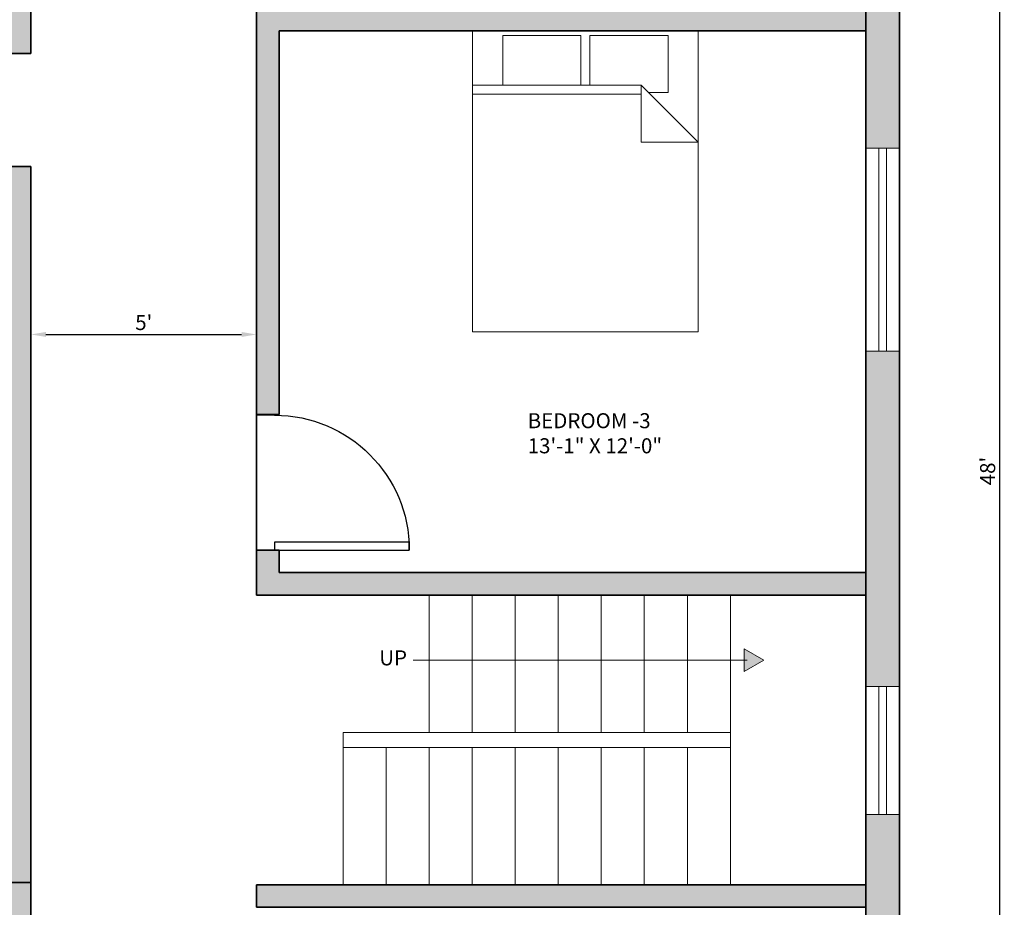
# Model space of a CAD drawing. Units: inches. Extents: x -91 to 518, y -600 to 105.
# Tile 3 of 4: x 248 to 509, y -391 to -155. Entities that reach past the tile are written whole.
import ezdxf

# ---------------------------------------------------------------- set-up
doc = ezdxf.new("R2010")
doc.units = ezdxf.units.IN
for name, color, linetype, lineweight in [('A-ANNO-DIMS', 2, 'Continuous', 18), ('A-ANNO-SYMB', 7, 'Continuous', 18), ('A-ANNO-TEXT', 7, 'Continuous', 18), ('A-AREA-IDEN', 7, 'Continuous', 18), ('A-DOOR', 4, 'Continuous', 25), ('A-FLOR-STRS', 7, 'Continuous', 18), ('A-FURN', 8, 'Continuous', 18), ('A-GLAZ', 6, 'Continuous', 18), ('A-WALL', 7, 'Continuous', 35), ('A-WALL-PATT', 251, 'Continuous', 13)]:
    doc.layers.add(name, color=color, linetype=linetype, lineweight=lineweight)
doc.styles.get("Standard").update_dxf_attribs({"font": 'arial.ttf'})
doc.dimstyles.new('ISO-25', dxfattribs={"dimtxt": 4, "dimasz": 4, "dimexe": 1.25, "dimexo": 0.625, "dimtad": 1, "dimlunit": 3, "dimtxsty": 'Standard', "dimcen": 2.5, "dimadec": 0, "dimazin": 0, "dimtfac": 1, "dimtmove": 0, "dimatfit": 3, "dimfxl": 1, "dimfxlon": 1, "dimarcsym": 0})

# ---------------------------------------------------------------- blocks, each defined once
blk = doc.blocks.new('*U2')
for p, q in [((0, 0), (0, -100)), ((750, 0), (750, -100))]:
    blk.add_line(p, q)
blk.add_lwpolyline([(0, 0), (0, 750), (43.75, 750), (43.75, 0)], close=True)
blk.add_arc((0, 0), 750, 0, 90)
blk = doc.blocks.new('Bed - Queen')
for p, q in [((0, -80.00003), (0, 0)), ((0, 0), (59.99999, 0)), ((59.99999, 0), (59.99999, -80.00003)), ((7.99999, -1.2), (28.79998, -1.2)), ((7.99999, -14.4), (7.99999, -1.2)), ((28.79998, -1.2), (28.79998, -14.4)), ((31.19999, -1.2), (51.99999, -1.2)), ((31.19999, -14.4), (31.19999, -1.2)), ((51.99999, -1.2), (51.99999, -16.4)), ((0, -14.4), (44.8, -14.4)), ((59.99999, -29.6), (44.8, -14.4)), ((44.8, -14.4), (44.8, -29.6)), ((44.8, -16.8), (0, -16.8)), ((51.99999, -16.4), (46.79936, -16.4)), ((44.8, -29.6), (59.99999, -29.6)), ((59.99999, -80.00003), (0, -80.00003))]:
    blk.add_line(p, q)
blk = doc.blocks.new('*D8')
at = {"layer": 'A-ANNO-DIMS', "color": 0, "lineweight": -2, "transparency": 16777216}
for p, q in [((250.54, -239), (250.54, -237.75)), ((310.54, -239), (310.54, -237.75)), ((254.54, -239), (306.54, -239))]:
    blk.add_line(p, q, dxfattribs=at)
at = {"layer": 'A-ANNO-DIMS', "color": 0, "transparency": 16777216}
for points in [[(254.54, -238.33), (254.54, -239.66), (250.54, -239)], [(306.54, -238.33), (306.54, -239.66), (310.54, -239)]]:
    blk.add_solid(points, dxfattribs=at)
at = {"layer": 'Defpoints', "color": 0, "transparency": 16777216}
for p in [(250.54, -239), (310.54, -239), (310.54, -239)]:
    blk.add_point(p, dxfattribs=at)
at = {"layer": 'A-ANNO-DIMS', "color": 0, "transparency": 16777216, "insert": (280.54, -236.34), "char_height": 4, "attachment_point": 5}
blk.add_mtext("5'", dxfattribs=at)
blk = doc.blocks.new('*D10')
at = {"layer": 'A-ANNO-DIMS', "color": 0, "lineweight": -2, "transparency": 16777216}
for p, q in [((507.14, 12.69), (509.39, 12.69)), ((508.14, 8.69), (508.14, -559.31)), ((507.14, -563.31), (509.39, -563.31))]:
    blk.add_line(p, q, dxfattribs=at)
at = {"layer": 'A-ANNO-DIMS', "color": 0, "transparency": 16777216}
for points in [[(507.48, 8.69), (508.81, 8.69), (508.14, 12.69)], [(507.48, -559.31), (508.81, -559.31), (508.14, -563.31)]]:
    blk.add_solid(points, dxfattribs=at)
at = {"layer": 'Defpoints', "color": 0, "transparency": 16777216}
for p in [(481.54, 12.69), (481.54, -563.31), (508.14, -563.31)]:
    blk.add_point(p, dxfattribs=at)
at = {"layer": 'A-ANNO-DIMS', "color": 0, "transparency": 16777216, "insert": (505.48, -275.31), "char_height": 4, "attachment_point": 5, "rotation": 90}
blk.add_mtext("48'", dxfattribs=at)
blk = doc.blocks.new('WIN-54IN')
for p, q in [((0, 5.5), (54, 5.5)), ((0, 3.5), (54, 3.5))]:
    blk.add_line(p, q)
blk.add_lwpolyline([(0, 9), (54, 9), (54, 0), (0, 0)], close=True)
blk = doc.blocks.new('WIN-34IN')
for p, q in [((0, 5.5), (34, 5.5)), ((0, 3.5), (34, 3.5))]:
    blk.add_line(p, q)
blk.add_lwpolyline([(0, 9), (34, 9), (34, 0), (0, 0)], close=True)
blk = doc.blocks.new('*D35')
at = {"layer": 'A-ANNO-DIMS', "color": 0, "lineweight": -2, "transparency": 16777216}
for p, q in [((-81.99, -381.31), (-81.99, -377.31)), ((-80.99, -385.31), (-83.24, -385.31)), ((-81.99, -385.31), (-81.99, -391.31)), ((-80.99, -391.31), (-83.24, -391.31)), ((-81.99, -395.31), (-81.99, -411.19))]:
    blk.add_line(p, q, dxfattribs=at)
at = {"layer": 'A-ANNO-DIMS', "color": 0, "transparency": 16777216}
for points in [[(-82.66, -381.31), (-81.32, -381.31), (-81.99, -385.31)], [(-82.66, -395.31), (-81.32, -395.31), (-81.99, -391.31)]]:
    blk.add_solid(points, dxfattribs=at)
at = {"layer": 'Defpoints', "color": 0, "transparency": 16777216}
for p in [(310.54, -385.31), (-81.99, -391.31), (310.54, -391.31)]:
    blk.add_point(p, dxfattribs=at)
at = {"layer": 'A-ANNO-DIMS', "color": 0, "transparency": 16777216, "insert": (-84.66, -405.25), "char_height": 4, "attachment_point": 5, "rotation": 90}
blk.add_mtext('0\'-6"', dxfattribs=at)
blk = doc.blocks.new('*D36')
at = {"layer": 'A-ANNO-DIMS', "color": 0, "lineweight": -2, "transparency": 16777216}
for p, q in [((-80.99, -308.31), (-83.24, -308.31)), ((-81.99, -381.31), (-81.99, -312.31)), ((-80.99, -385.31), (-83.24, -385.31))]:
    blk.add_line(p, q, dxfattribs=at)
at = {"layer": 'A-ANNO-DIMS', "color": 0, "transparency": 16777216}
for points in [[(-82.66, -312.31), (-81.32, -312.31), (-81.99, -308.31)], [(-82.66, -381.31), (-81.32, -381.31), (-81.99, -385.31)]]:
    blk.add_solid(points, dxfattribs=at)
at = {"layer": 'Defpoints', "color": 0, "transparency": 16777216}
for p in [(-81.99, -308.31), (472.54, -308.31), (472.54, -385.31)]:
    blk.add_point(p, dxfattribs=at)
at = {"layer": 'A-ANNO-DIMS', "color": 0, "transparency": 16777216, "insert": (-84.66, -346.81), "char_height": 4, "attachment_point": 5, "rotation": 90}
blk.add_mtext('6\'-5"', dxfattribs=at)
blk = doc.blocks.new('*D38')
at = {"layer": 'A-ANNO-DIMS', "color": 0, "lineweight": -2, "transparency": 16777216}
for p, q in [((449.61, 95.59), (449.61, 97.84)), ((472.54, 95.59), (472.54, 97.84)), ((453.61, 96.59), (468.54, 96.59))]:
    blk.add_line(p, q, dxfattribs=at)
at = {"layer": 'A-ANNO-DIMS', "color": 0, "transparency": 16777216}
for points in [[(453.61, 97.25), (453.61, 95.92), (449.61, 96.59)], [(468.54, 97.25), (468.54, 95.92), (472.54, 96.59)]]:
    blk.add_solid(points, dxfattribs=at)
at = {"layer": 'Defpoints', "color": 0, "transparency": 16777216}
for p in [(472.54, 96.59), (449.61, -434.96), (472.54, -434.96)]:
    blk.add_point(p, dxfattribs=at)
at = {"layer": 'A-ANNO-DIMS', "color": 0, "transparency": 16777216, "insert": (461.08, 99.22), "char_height": 4, "attachment_point": 5}
blk.add_mtext('1\'-11"', dxfattribs=at)
blk = doc.blocks.new('*D46')
at = {"layer": 'A-ANNO-DIMS', "color": 0, "lineweight": -2, "transparency": 16777216}
for p, q in [((250.54, -595.36), (250.54, -597.61)), ((254.54, -596.36), (270.34, -596.36)), ((274.34, -595.36), (274.34, -597.61))]:
    blk.add_line(p, q, dxfattribs=at)
at = {"layer": 'A-ANNO-DIMS', "color": 0, "transparency": 16777216}
for points in [[(254.54, -595.69), (254.54, -597.02), (250.54, -596.36)], [(270.34, -595.69), (270.34, -597.02), (274.34, -596.36)]]:
    blk.add_solid(points, dxfattribs=at)
at = {"layer": 'Defpoints', "color": 0, "transparency": 16777216}
for p in [(250.54, 3.69), (274.34, 3.69), (274.34, -596.36)]:
    blk.add_point(p, dxfattribs=at)
at = {"layer": 'A-ANNO-DIMS', "color": 0, "transparency": 16777216, "insert": (262.44, -593.69), "char_height": 4, "attachment_point": 5}
blk.add_mtext('2\'-0"', dxfattribs=at)
blk = doc.blocks.new('*D48')
at = {"layer": 'A-ANNO-DIMS', "color": 0, "lineweight": -2, "transparency": 16777216}
for p, q in [((-80.99, -158.31), (-83.24, -158.31)), ((-81.99, -162.31), (-81.99, -185.45)), ((-80.99, -189.45), (-83.24, -189.45))]:
    blk.add_line(p, q, dxfattribs=at)
at = {"layer": 'A-ANNO-DIMS', "color": 0, "transparency": 16777216}
for points in [[(-82.66, -162.31), (-81.32, -162.31), (-81.99, -158.31)], [(-82.66, -185.45), (-81.32, -185.45), (-81.99, -189.45)]]:
    blk.add_solid(points, dxfattribs=at)
at = {"layer": 'Defpoints', "color": 0, "transparency": 16777216}
for p in [(472.54, -158.31), (-81.99, -189.45), (472.54, -189.45)]:
    blk.add_point(p, dxfattribs=at)
at = {"layer": 'A-ANNO-DIMS', "color": 0, "transparency": 16777216, "insert": (-84.62, -173.88), "char_height": 4, "attachment_point": 5, "rotation": 90}
blk.add_mtext('2\'-7"', dxfattribs=at)
blk = doc.blocks.new('*D49')
at = {"layer": 'A-ANNO-DIMS', "color": 0, "lineweight": -2, "transparency": 16777216}
for p, q in [((-80.99, -308.31), (-83.24, -308.31)), ((-81.99, -312.31), (-81.99, -328.59)), ((-80.99, -332.59), (-83.24, -332.59))]:
    blk.add_line(p, q, dxfattribs=at)
at = {"layer": 'A-ANNO-DIMS', "color": 0, "transparency": 16777216}
for points in [[(-82.66, -312.31), (-81.32, -312.31), (-81.99, -308.31)], [(-82.66, -328.59), (-81.32, -328.59), (-81.99, -332.59)]]:
    blk.add_solid(points, dxfattribs=at)
at = {"layer": 'Defpoints', "color": 0, "transparency": 16777216}
for p in [(472.54, -308.31), (-81.99, -332.59), (472.54, -332.59)]:
    blk.add_point(p, dxfattribs=at)
at = {"layer": 'A-ANNO-DIMS', "color": 0, "transparency": 16777216, "insert": (-84.68, -320.45), "char_height": 4, "attachment_point": 5, "rotation": 90}
blk.add_mtext('2\'-0 1/2"', dxfattribs=at)
blk = doc.blocks.new('*D51')
at = {"layer": 'A-ANNO-DIMS', "color": 0, "lineweight": -2, "transparency": 16777216}
for p, q in [((250.54, 95.59), (250.54, 97.84)), ((269.18, 95.59), (269.18, 97.84)), ((254.54, 96.59), (265.18, 96.59)), ((269.18, 96.59), (294.01, 96.59))]:
    blk.add_line(p, q, dxfattribs=at)
at = {"layer": 'A-ANNO-DIMS', "color": 0, "transparency": 16777216}
for points in [[(254.54, 97.25), (254.54, 95.92), (250.54, 96.59)], [(265.18, 97.25), (265.18, 95.92), (269.18, 96.59)]]:
    blk.add_solid(points, dxfattribs=at)
at = {"layer": 'Defpoints', "color": 0, "transparency": 16777216}
for p in [(269.18, 96.59), (250.54, -554.31), (269.18, -554.26)]:
    blk.add_point(p, dxfattribs=at)
at = {"layer": 'A-ANNO-DIMS', "color": 0, "transparency": 16777216, "insert": (283.6, 99.28), "char_height": 4, "attachment_point": 5}
blk.add_mtext('1\'-6 1/2"', dxfattribs=at)
blk = doc.blocks.new('*D57')
at = {"layer": 'A-ANNO-DIMS', "color": 0, "lineweight": -2, "transparency": 16777216}
for p, q in [((-80.99, -348.81), (-83.24, -348.81)), ((-81.99, -381.31), (-81.99, -352.81)), ((-80.99, -385.31), (-83.24, -385.31))]:
    blk.add_line(p, q, dxfattribs=at)
at = {"layer": 'A-ANNO-DIMS', "color": 0, "transparency": 16777216}
for points in [[(-82.66, -352.81), (-81.32, -352.81), (-81.99, -348.81)], [(-82.66, -381.31), (-81.32, -381.31), (-81.99, -385.31)]]:
    blk.add_solid(points, dxfattribs=at)
at = {"layer": 'Defpoints', "color": 0, "transparency": 16777216}
for p in [(-81.99, -348.81), (333.53, -348.81), (333.53, -385.31)]:
    blk.add_point(p, dxfattribs=at)
at = {"layer": 'A-ANNO-DIMS', "color": 0, "transparency": 16777216, "insert": (-84.68, -367.06), "char_height": 4, "attachment_point": 5, "rotation": 90}
blk.add_mtext('3\'-0 1/2"', dxfattribs=at)
blk = doc.blocks.new('*D58')
at = {"layer": 'A-ANNO-DIMS', "color": 0, "lineweight": -2, "transparency": 16777216}
for p, q in [((375.09, 95.59), (375.09, 97.84)), ((400.72, 95.59), (400.72, 97.84)), ((379.09, 96.59), (396.72, 96.59))]:
    blk.add_line(p, q, dxfattribs=at)
at = {"layer": 'A-ANNO-DIMS', "color": 0, "transparency": 16777216}
for points in [[(379.09, 97.25), (379.09, 95.92), (375.09, 96.59)], [(396.72, 97.25), (396.72, 95.92), (400.72, 96.59)]]:
    blk.add_solid(points, dxfattribs=at)
at = {"layer": 'Defpoints', "color": 0, "transparency": 16777216}
for p in [(400.72, 96.59), (375.09, -530.31), (400.72, -533.48)]:
    blk.add_point(p, dxfattribs=at)
at = {"layer": 'A-ANNO-DIMS', "color": 0, "transparency": 16777216, "insert": (387.9, 99.28), "char_height": 4, "attachment_point": 5}
blk.add_mtext('2\'-1 1/2"', dxfattribs=at)

msp = doc.modelspace()

# ---------------------------------------------------------------- hatches: boundary and pattern name
at = {"layer": 'A-ANNO-SYMB'}
h = msp.add_hatch(color=256, dxfattribs=at)
h.dxf.hatch_style = 1
h.paths.add_polyline_path([(445.404, -325.614), (440.208, -322.614), (440.208, -328.614)])
at = {"layer": 'A-WALL-PATT'}
h = msp.add_hatch(color=256, dxfattribs=at)
h.dxf.hatch_style = 1
h.paths.add_polyline_path([(10.544, 3.693), (34.462, 3.693), (34.462, 12.693), (1.544, 12.693), (1.544, -180.878), (10.544, -180.878)])
h.paths.add_polyline_path([(46.544, -92.307), (10.544, -92.307), (10.544, -98.307), (46.544, -98.307)])
h.paths.add_polyline_path([(130.381, 12.693), (52.462, 12.693), (52.462, 3.693), (82.544, 3.693), (88.544, 3.693), (130.381, 3.693)])
h.paths.add_polyline_path([(88.544, 3.693), (82.544, 3.693), (82.544, -92.307), (76.544, -92.307), (76.544, -94.37), (76.544, -98.307), (82.544, -98.307), (82.544, -106.057), (85.522, -106.057), (88.544, -106.057)])
h.paths.add_polyline_path([(250.544, -146.307), (245.772, -146.307), (244.544, -146.307), (244.544, -152.307), (88.544, -152.307), (88.544, -141.744), (85.718, -141.744), (82.544, -141.744), (82.544, -152.307), (10.544, -152.307), (10.544, -158.307), (88.544, -158.307), (118.544, -158.307), (118.544, -164.307), (120.607, -164.307), (124.544, -164.307), (124.544, -158.307), (244.544, -158.307), (244.544, -164.307), (250.544, -164.307)])
h.paths.add_polyline_path([(274.341, 12.693), (184.381, 12.693), (184.381, 3.693), (244.544, 3.693), (250.544, 3.693), (274.341, 3.693)])
h.paths.add_polyline_path([(250.544, 3.693), (244.544, 3.693), (244.544, -110.307), (250.544, -110.307), (250.544, -98.307), (310.544, -98.307), (310.544, -110.307), (316.544, -110.307), (316.544, -86.517), (312.607, -86.517), (310.544, -86.517), (310.544, -92.307), (250.544, -92.307)])
h.paths.add_polyline_path([(481.544, 12.693), (292.341, 12.693), (292.341, 3.693), (310.544, 3.693), (316.544, 3.693), (472.544, 3.693), (472.544, -34.129), (481.544, -34.129)])
h.paths.add_polyline_path([(316.544, 3.693), (310.544, 3.693), (310.544, -56.517), (316.544, -56.517)], flags=17)
h.paths.add_polyline_path([(481.544, -88.129), (472.544, -88.129), (472.544, -189.451), (481.544, -189.451)])
h.paths.add_polyline_path([(472.544, -152.307), (316.544, -152.307), (316.544, -146.307), (315.319, -146.307), (310.544, -146.307), (310.544, -260.307), (316.544, -260.307), (316.544, -158.307), (472.544, -158.307)])
h.paths.add_polyline_path([(481.544, -243.451), (472.544, -243.451), (472.544, -308.307), (472.544, -332.593), (481.544, -332.593)])
h.paths.add_polyline_path([(472.544, -302.307), (316.544, -302.307), (316.544, -296.307), (315.322, -296.307), (310.544, -296.307), (310.544, -308.307), (472.544, -308.307)])
h.paths.add_polyline_path([(481.544, -366.593), (472.544, -366.593), (472.544, -385.307), (472.544, -456.136), (481.544, -456.136)])
h.paths.add_polyline_path([(472.544, -385.307), (310.544, -385.307), (310.544, -391.307), (472.544, -391.307)])
h.paths.add_polyline_path([(481.544, -510.136), (472.544, -510.136), (472.544, -554.307), (323.185, -554.307), (323.185, -563.307), (481.544, -563.307)])
h.paths.add_polyline_path([(250.544, -384.724), (229.645, -384.724), (229.645, -393.724), (241.544, -393.724), (241.544, -563.307), (269.185, -563.307), (269.185, -554.307), (250.544, -554.307)])
h.paths.add_polyline_path([(195.645, -384.724), (133.7, -384.724), (133.7, -393.724), (195.645, -393.724)])
h.paths.add_polyline_path([(99.7, -384.724), (61.544, -384.724), (61.544, -391.562), (61.335, -393.724), (77.042, -393.724), (99.7, -393.724)])
h.paths.add_polyline_path([(10.544, -264.014), (1.544, -264.014), (1.544, -330.048), (10.544, -330.048)])
h.paths.add_polyline_path([(10.544, -198.878), (1.544, -198.878), (1.544, -230.014), (10.544, -230.014)])
h.paths.add_polyline_path([(208.544, -218.307), (124.544, -218.307), (124.544, -194.307), (118.544, -194.307), (118.544, -218.307), (10.544, -218.307), (10.544, -224.307), (118.544, -224.307), (124.544, -224.307), (208.544, -224.307)])
h.paths.add_polyline_path([(250.544, -194.307), (244.544, -194.307), (244.544, -218.307), (238.544, -218.307), (238.544, -224.307), (244.544, -224.307), (244.544, -384.724), (250.544, -384.724)])

# ---------------------------------------------------------------- linework, layer by layer
at = {"layer": 'A-ANNO-SYMB'}
msp.add_line((352.193, -325.641), (441.021, -325.641), dxfattribs=at)
msp.add_lwpolyline([(440.208, -322.614), (440.208, -328.614), (445.404, -325.614)], close=True, dxfattribs=at)
at = {"layer": 'A-FLOR-STRS'}
for p, q in [((356.424, -308.307), (356.424, -344.807)), ((367.87, -308.307), (367.87, -344.807)), ((379.315, -308.307), (379.315, -344.807)), ((390.761, -308.307), (390.761, -344.807)), ((402.207, -308.307), (402.207, -344.807)), ((413.652, -308.307), (413.652, -344.807)), ((425.098, -308.307), (425.098, -344.807)), ((436.544, -308.307), (436.544, -344.807)), ((333.532, -385.307), (333.532, -344.807)), ((333.532, -344.807), (436.544, -344.807)), ((436.544, -344.807), (436.544, -348.807)), ((333.532, -348.807), (436.544, -348.807)), ((333.532, -348.807), (333.532, -385.307)), ((344.978, -348.807), (344.978, -385.307)), ((356.424, -348.807), (356.424, -385.307)), ((367.87, -348.807), (367.87, -385.307)), ((379.315, -348.807), (379.315, -385.307)), ((390.761, -348.807), (390.761, -385.307)), ((402.207, -348.807), (402.207, -385.307)), ((413.652, -348.807), (413.652, -385.307)), ((425.098, -348.807), (425.098, -385.307)), ((436.544, -348.807), (436.544, -385.307))]:
    msp.add_line(p, q, dxfattribs=at)
at = {"layer": 'A-WALL'}
for p, q in [((481.544, 12.693), (481.544, -563.307)), ((472.544, 3.693), (472.544, -308.307)), ((250.544, -164.307), (250.544, -98.307)), ((310.544, -308.307), (310.544, -98.307)), ((316.544, -158.307), (472.544, -158.307)), ((316.544, -260.307), (316.544, -158.307)), ((244.544, -164.307), (250.544, -164.307)), ((244.544, -194.307), (250.544, -194.307)), ((250.544, -554.307), (250.544, -194.307)), ((316.544, -260.307), (310.544, -260.307)), ((316.544, -296.307), (310.544, -296.307)), ((316.544, -302.307), (316.544, -296.307)), ((316.544, -302.307), (472.544, -302.307)), ((310.544, -308.307), (472.544, -308.307)), ((472.544, -308.307), (472.544, -385.307)), ((250.544, -384.724), (61.544, -384.724)), ((310.544, -391.307), (310.544, -385.307)), ((472.544, -385.307), (310.544, -385.307)), ((472.544, -385.307), (472.544, -554.307)), ((472.544, -391.307), (310.544, -391.307))]:
    msp.add_line(p, q, dxfattribs=at)

# ---------------------------------------------------------------- block references
at = {"layer": 'A-DOOR', "xscale": -0.047783582079683, "yscale": 0.047783582079683, "zscale": 0.047783582079683, "rotation": 270}
msp.add_blockref('*U2', (315.322, -296.307), dxfattribs=at)
at = {"layer": 'A-FURN'}
msp.add_blockref('Bed - Queen', (367.991, -158.307), dxfattribs=at)
at = {"layer": 'A-GLAZ'}
for name, p, rotation in [('WIN-54IN', (472.544, -189.452), 269.9999999999999), ('WIN-34IN', (472.544, -332.593), 270.0000000000002)]:
    msp.add_blockref(name, p, dxfattribs=dict(at, rotation=rotation))

# ---------------------------------------------------------------- texts
at = {"layer": 'A-ANNO-TEXT', "insert": (343.161, -322.986), "char_height": 4, "attachment_point": 1}
msp.add_mtext_dynamic_manual_height_columns('UP', width=6.4852, gutter_width=12.5, heights=[0], dxfattribs=at)
at = {"layer": 'A-AREA-IDEN', "insert": (382.644, -259.929), "char_height": 4, "attachment_point": 1}
msp.add_mtext_dynamic_manual_height_columns('BEDROOM -3\\P13\'-1" X 12\'-0"', width=82.10685, gutter_width=12.5, heights=[0], dxfattribs=at)

# ---------------------------------------------------------------- dimensions: what is measured, and where the dimension line sits
at = {"layer": 'A-ANNO-DIMS'}
for base, p1, p2, override, picture, middle in [((269.185, 96.588), (250.544, -554.307), (269.185, -554.258), {"dimdec": 1, "dimlfac": 1, "dimrnd": 0, "dimzin": 1, "dimdsep": 46, "dimlunit": 4, "dimfrac": 2}, '*D51', (283.598, 99.281)), ((400.722, 96.588), (375.087, -530.307), (400.722, -533.48), {"dimdec": 1, "dimlfac": 1, "dimrnd": 0, "dimzin": 1, "dimdsep": 46, "dimlunit": 4, "dimfrac": 2}, '*D58', (387.904, 99.281)), ((472.544, 96.588), (449.608, -434.957), (472.544, -434.957), {"dimdec": 1, "dimlfac": 1, "dimrnd": 0, "dimzin": 1, "dimdsep": 46, "dimlunit": 4, "dimfrac": 2}, '*D38', (461.076, 99.221)), ((274.341, -596.357), (250.544, 3.693), (274.341, 3.693), {"dimdec": 1, "dimlfac": 1, "dimrnd": 0, "dimzin": 1, "dimdsep": 46, "dimlunit": 4, "dimfrac": 2}, '*D46', (262.442, -593.69)), ((310.544, -238.997), (250.544, -238.997), (310.544, -238.997), {"dimclrd": 0, "dimclre": 0, "dimclrt": 0}, '*D8', (280.544, -236.338))]:
    dim = msp.add_linear_dim(base=base, p1=p1, p2=p2, dimstyle='ISO-25', override=override, dxfattribs=at)
    dim.commit()
    dim.dimension.update_dxf_attribs({"geometry": picture, "text_midpoint": middle})
for base, p1, p2, override, picture, middle in [((508.145, -563.307), (481.544, 12.693), (481.544, -563.307), {"dimclrd": 0, "dimclre": 0, "dimclrt": 0}, '*D10', (505.477, -275.307)), ((-81.989, -189.451), (472.544, -158.307), (472.544, -189.451), {"dimdec": 1, "dimlfac": 1, "dimrnd": 0, "dimzin": 1, "dimdsep": 46, "dimlunit": 4, "dimfrac": 2}, '*D48', (-84.622, -173.879)), ((-81.989, -332.593), (472.544, -308.307), (472.544, -332.593), {"dimdec": 1, "dimlfac": 1, "dimrnd": 0, "dimzin": 1, "dimdsep": 46, "dimlunit": 4, "dimfrac": 2}, '*D49', (-84.682, -320.45)), ((-81.989, -308.307), (472.544, -385.307), (472.544, -308.307), {"dimdec": 1, "dimlfac": 1, "dimrnd": 0, "dimzin": 1, "dimdsep": 46, "dimlunit": 4, "dimfrac": 2}, '*D36', (-84.656, -346.807)), ((-81.989, -348.807), (333.532, -385.307), (333.532, -348.807), {"dimdec": 1, "dimlfac": 1, "dimrnd": 0, "dimzin": 1, "dimdsep": 46, "dimlunit": 4, "dimfrac": 2}, '*D57', (-84.683, -367.057)), ((-81.989, -391.307), (310.544, -385.307), (310.544, -391.307), {"dimdec": 1, "dimlfac": 1, "dimrnd": 0, "dimzin": 1, "dimdsep": 46, "dimlunit": 4, "dimfrac": 2}, '*D35', (-84.656, -405.249))]:
    dim = msp.add_linear_dim(base=base, p1=p1, p2=p2, angle=90, dimstyle='ISO-25', override=override, dxfattribs=at)
    dim.commit()
    dim.dimension.update_dxf_attribs({"geometry": picture, "text_midpoint": middle})

doc.saveas('drawing.dxf')
